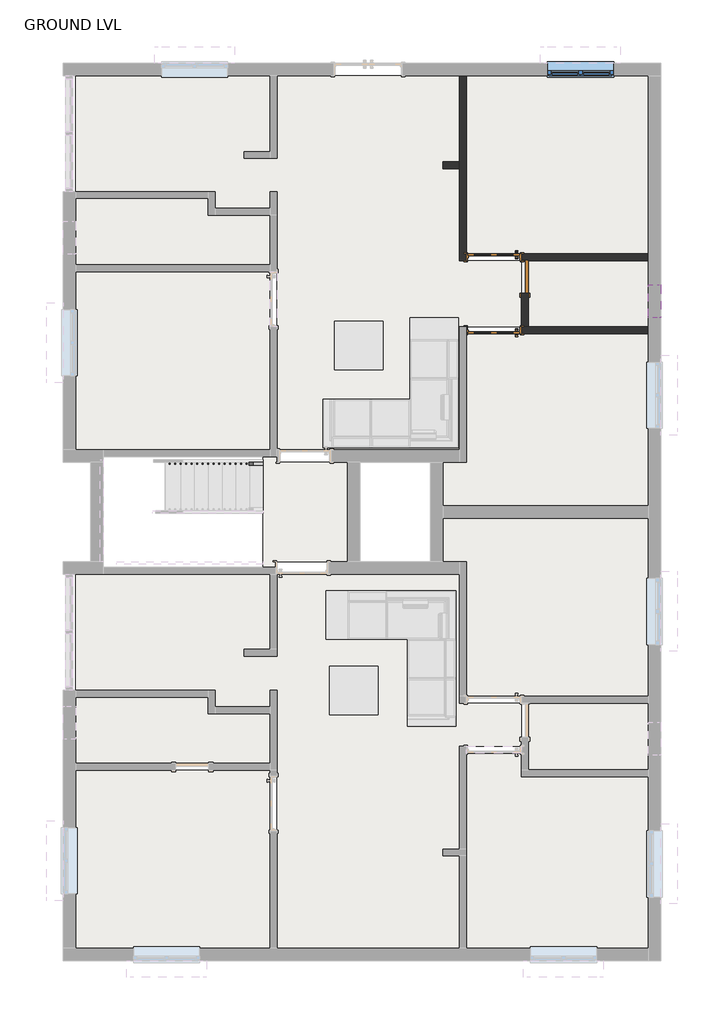
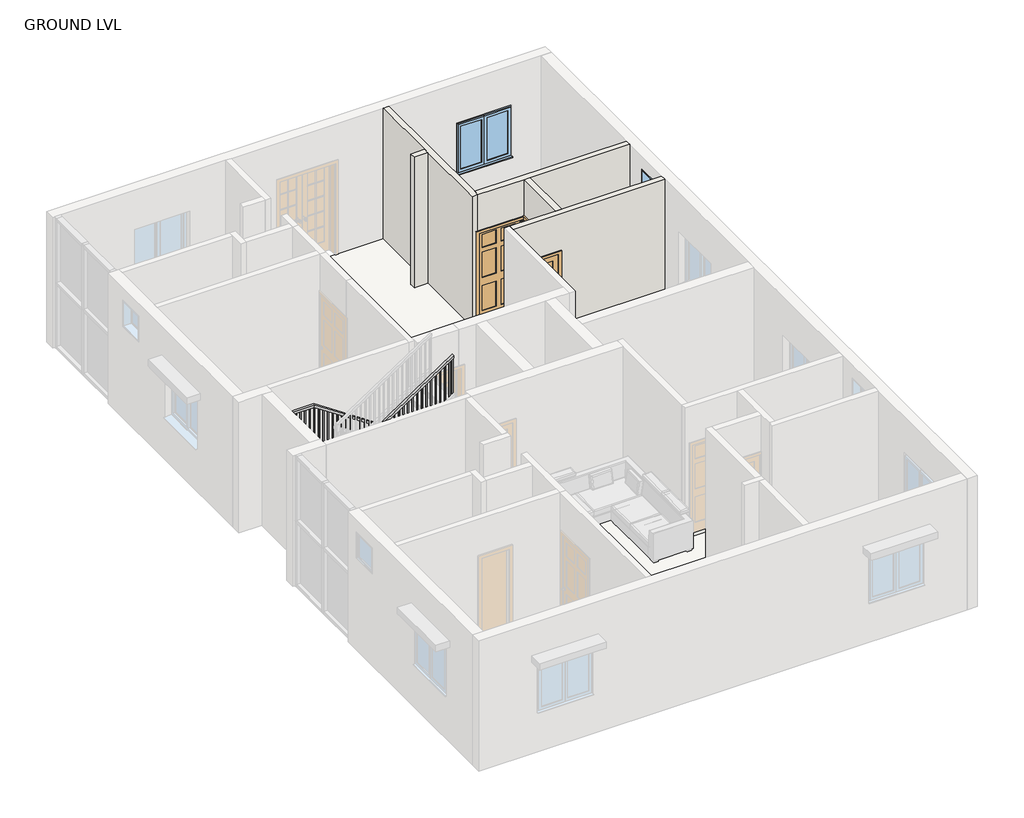
# One storey, part 3 of 4: 5 walls, 4 slabs, 3 doors, 2 windows, 1 railing.
"""IFC4 building model written with IfcOpenShell, lengths in millimetres."""

from ifc_helpers import new_model, si_unit, frame, origin, place, context, project, spatial, polyline, outline, extrude, faceted_brep, transform, mapped, element, save
from components import door_6a452240, door_3d68aebc, single_flush_flush_door_2_x_7_931cabab, window_80340324, w2_windows_4_x_4_9dec5fc7

model = new_model("IFC4")

# Units and contexts
model_context = context("Model", 3, world=origin())
ifc_project = project(units=[si_unit("LENGTHUNIT", "METRE", prefix="MILLI")], contexts=[model_context])

# Site, building, storey
site = spatial("IfcSite", under=ifc_project)
building = spatial("IfcBuilding", under=site)
storey = spatial("IfcBuildingStorey", under=building, Name="GROUND LVL", Elevation=3048.0)

# Doors
placement = place(None, origin())
door_shape = door_6a452240(model_context)
element("IfcDoor", 1, ObjectType="Door-Interior-Single-6_Panel-Wood : interior door 3' 4\" x 7'", at=placement, inside=storey, context=model_context, shape_type="MappedRepresentation", body=[
    mapped(door_shape, transform((1493.7987798, 9705.7059003, 3048.0), x_axis=(-1.0, 0.0, 0.0), y_axis=(0.0, -1.0, 0.0), z_axis=(0.0, 0.0, 1.0))),
])
door_2_shape = door_3d68aebc(model_context)
element("IfcDoor", 2, ObjectType="Door-Interior-Single-6_Panel-Wood : interior door 3' 4\" x 7'", at=placement, inside=storey, context=model_context, shape_type="MappedRepresentation", body=[
    mapped(door_2_shape, transform((1493.7987798, 8353.1559003, 3048.0), x_axis=(-1.0, 0.0, 0.0), y_axis=(0.0, -1.0, 0.0), z_axis=(0.0, 0.0, 1.0))),
])
single_flush_flush_door_2_x_7_shape = single_flush_flush_door_2_x_7_931cabab(model_context)
element("IfcDoor", 3, ObjectType="Single-Flush : flush door 2' x 7'", at=placement, inside=storey, context=model_context, shape_type="MappedRepresentation", body=[
    mapped(single_flush_flush_door_2_x_7_shape, transform((2065.2987798, 9346.9309003, 3048.0), x_axis=(0.0, 1.0, 0.0), y_axis=(-1.0, 0.0, 0.0), z_axis=(0.0, 0.0, 1.0))),
])

# Railing
element("IfcRailing", 4, ObjectType="Handrail - Rectangular", at=placement, inside=storey, context=model_context, shape_type="SolidModel", body=[
    faceted_brep([(-2748.0012202, 5879.8309003, 4131.7333333), (-2748.0012202, 5879.8309003, 4070.6793317), (-2748.0012202, 5930.6309003, 4070.6793317), (-2748.0012202, 5930.6309003, 4131.7333333), (-4780.0012202, 5879.8309003, 5486.4), (-4795.3822226, 5879.8309003, 5435.6), (-4795.3822226, 5930.6309003, 5435.6), (-4780.0012202, 5930.6309003, 5486.4), (-5643.6012202, 5879.8309003, 5486.4), (-5643.6012202, 5879.8309003, 5435.6), (-5694.4012202, 5930.6309003, 5435.6), (-5694.4012202, 5930.6309003, 5486.4), (-5643.6012202, 4152.6309003, 5486.4), (-5643.6012202, 4152.6309003, 5435.6), (-5694.4012202, 4101.8309003, 5435.6), (-5694.4012202, 4101.8309003, 5486.4), (-5034.0012202, 4152.6309003, 5486.4), (-5018.6202178, 4152.6309003, 5435.6), (-5018.6202178, 4101.8309003, 5435.6), (-5034.0012202, 4101.8309003, 5486.4), (-2748.0012202, 4152.6309003, 7010.4), (-2748.0012202, 4101.8309003, 7010.4), (-2748.0012202, 4101.8309003, 6949.3459984), (-2748.0012202, 4152.6309003, 6949.3459984)], [[[0, 1, 2, 3]], [[1, 0, 4, 5]], [[2, 1, 5, 6]], [[3, 2, 6, 7]], [[0, 3, 7, 4]], [[5, 4, 8, 9]], [[6, 5, 9, 10]], [[7, 6, 10, 11]], [[4, 7, 11, 8]], [[9, 8, 12, 13]], [[10, 9, 13, 14]], [[11, 10, 14, 15]], [[8, 11, 15, 12]], [[13, 12, 16, 17]], [[14, 13, 17, 18]], [[15, 14, 18, 19]], [[12, 15, 19, 16]], [[20, 21, 22, 23]], [[17, 16, 20, 23]], [[18, 17, 23, 22]], [[19, 18, 22, 21]], [[16, 19, 21, 20]]]),
    extrude(outline(polyline([(6904.8959984, -2814.6762202), (6892.1959984, -2833.7262202), (5926.6666667, -2833.7262202), (5926.6666667, -2814.6762202), (6904.8959984, -2814.6762202)])), frame((0.0, 4117.7059003, 0.0), z_axis=(0.0, 1.0, 0.0), x_axis=(0.0, 0.0, 1.0)), (0.0, 0.0, 1.0), 19.05),
    extrude(outline(polyline([(6837.1626651, -2916.2762202), (6824.4626651, -2935.3262202), (5926.6666667, -2935.3262202), (5926.6666667, -2916.2762202), (6837.1626651, -2916.2762202)])), frame((0.0, 4117.7059003, 0.0), z_axis=(0.0, 1.0, 0.0), x_axis=(0.0, 0.0, 1.0)), (0.0, 0.0, 1.0), 19.05),
    extrude(outline(polyline([(6769.4293317, -3017.8762202), (6756.7293317, -3036.9262202), (5757.3333333, -3036.9262202), (5757.3333333, -3017.8762202), (6769.4293317, -3017.8762202)])), frame((0.0, 4117.7059003, 0.0), z_axis=(0.0, 1.0, 0.0), x_axis=(0.0, 0.0, 1.0)), (0.0, 0.0, 1.0), 19.05),
    extrude(outline(polyline([(6701.6959984, -3119.4762202), (6688.9959984, -3138.5262202), (5757.3333333, -3138.5262202), (5757.3333333, -3119.4762202), (6701.6959984, -3119.4762202)])), frame((0.0, 4117.7059003, 0.0), z_axis=(0.0, 1.0, 0.0), x_axis=(0.0, 0.0, 1.0)), (0.0, 0.0, 1.0), 19.05),
    extrude(outline(polyline([(6633.9626651, -3221.0762202), (6621.2626651, -3240.1262202), (5757.3333333, -3240.1262202), (5757.3333333, -3221.0762202), (6633.9626651, -3221.0762202)])), frame((0.0, 4117.7059003, 0.0), z_axis=(0.0, 1.0, 0.0), x_axis=(0.0, 0.0, 1.0)), (0.0, 0.0, 1.0), 19.05),
    extrude(outline(polyline([(6566.2293317, -3322.6762202), (6553.5293317, -3341.7262202), (5588.0, -3341.7262202), (5588.0, -3322.6762202), (6566.2293317, -3322.6762202)])), frame((0.0, 4117.7059003, 0.0), z_axis=(0.0, 1.0, 0.0), x_axis=(0.0, 0.0, 1.0)), (0.0, 0.0, 1.0), 19.05),
    extrude(outline(polyline([(6498.4959984, -3424.2762202), (6485.7959984, -3443.3262202), (5588.0, -3443.3262202), (5588.0, -3424.2762202), (6498.4959984, -3424.2762202)])), frame((0.0, 4117.7059003, 0.0), z_axis=(0.0, 1.0, 0.0), x_axis=(0.0, 0.0, 1.0)), (0.0, 0.0, 1.0), 19.05),
    extrude(outline(polyline([(6430.7626651, -3525.8762202), (6418.0626651, -3544.9262202), (5418.6666667, -3544.9262202), (5418.6666667, -3525.8762202), (6430.7626651, -3525.8762202)])), frame((0.0, 4117.7059003, 0.0), z_axis=(0.0, 1.0, 0.0), x_axis=(0.0, 0.0, 1.0)), (0.0, 0.0, 1.0), 19.05),
    extrude(outline(polyline([(6363.0293317, -3627.4762202), (6350.3293317, -3646.5262202), (5418.6666667, -3646.5262202), (5418.6666667, -3627.4762202), (6363.0293317, -3627.4762202)])), frame((0.0, 4117.7059003, 0.0), z_axis=(0.0, 1.0, 0.0), x_axis=(0.0, 0.0, 1.0)), (0.0, 0.0, 1.0), 19.05),
    extrude(outline(polyline([(6295.2959984, -3729.0762202), (6282.5959984, -3748.1262202), (5418.6666667, -3748.1262202), (5418.6666667, -3729.0762202), (6295.2959984, -3729.0762202)])), frame((0.0, 4117.7059003, 0.0), z_axis=(0.0, 1.0, 0.0), x_axis=(0.0, 0.0, 1.0)), (0.0, 0.0, 1.0), 19.05),
    extrude(outline(polyline([(6227.5626651, -3830.6762202), (6214.8626651, -3849.7262202), (5249.3333333, -3849.7262202), (5249.3333333, -3830.6762202), (6227.5626651, -3830.6762202)])), frame((0.0, 4117.7059003, 0.0), z_axis=(0.0, 1.0, 0.0), x_axis=(0.0, 0.0, 1.0)), (0.0, 0.0, 1.0), 19.05),
    extrude(outline(polyline([(6159.8293317, -3932.2762202), (6147.1293317, -3951.3262202), (5249.3333333, -3951.3262202), (5249.3333333, -3932.2762202), (6159.8293317, -3932.2762202)])), frame((0.0, 4117.7059003, 0.0), z_axis=(0.0, 1.0, 0.0), x_axis=(0.0, 0.0, 1.0)), (0.0, 0.0, 1.0), 19.05),
    extrude(outline(polyline([(6092.0959984, -4033.8762202), (6079.3959984, -4052.9262202), (5080.0, -4052.9262202), (5080.0, -4033.8762202), (6092.0959984, -4033.8762202)])), frame((0.0, 4117.7059003, 0.0), z_axis=(0.0, 1.0, 0.0), x_axis=(0.0, 0.0, 1.0)), (0.0, 0.0, 1.0), 19.05),
    extrude(outline(polyline([(6024.3626651, -4135.4762202), (6011.6626651, -4154.5262202), (5080.0, -4154.5262202), (5080.0, -4135.4762202), (6024.3626651, -4135.4762202)])), frame((0.0, 4117.7059003, 0.0), z_axis=(0.0, 1.0, 0.0), x_axis=(0.0, 0.0, 1.0)), (0.0, 0.0, 1.0), 19.05),
    extrude(outline(polyline([(5956.6293317, -4237.0762202), (5943.9293317, -4256.1262202), (5080.0, -4256.1262202), (5080.0, -4237.0762202), (5956.6293317, -4237.0762202)])), frame((0.0, 4117.7059003, 0.0), z_axis=(0.0, 1.0, 0.0), x_axis=(0.0, 0.0, 1.0)), (0.0, 0.0, 1.0), 19.05),
    extrude(outline(polyline([(5888.8959984, -4338.6762202), (5876.1959984, -4357.7262202), (4910.6666667, -4357.7262202), (4910.6666667, -4338.6762202), (5888.8959984, -4338.6762202)])), frame((0.0, 4117.7059003, 0.0), z_axis=(0.0, 1.0, 0.0), x_axis=(0.0, 0.0, 1.0)), (0.0, 0.0, 1.0), 19.05),
    extrude(outline(polyline([(5821.1626651, -4440.2762202), (5808.4626651, -4459.3262202), (4910.6666667, -4459.3262202), (4910.6666667, -4440.2762202), (5821.1626651, -4440.2762202)])), frame((0.0, 4117.7059003, 0.0), z_axis=(0.0, 1.0, 0.0), x_axis=(0.0, 0.0, 1.0)), (0.0, 0.0, 1.0), 19.05),
    extrude(outline(polyline([(5753.4293317, -4541.8762202), (5740.7293317, -4560.9262202), (4741.3333333, -4560.9262202), (4741.3333333, -4541.8762202), (5753.4293317, -4541.8762202)])), frame((0.0, 4117.7059003, 0.0), z_axis=(0.0, 1.0, 0.0), x_axis=(0.0, 0.0, 1.0)), (0.0, 0.0, 1.0), 19.05),
    extrude(outline(polyline([(5685.6959984, -4643.4762202), (5672.9959984, -4662.5262202), (4741.3333333, -4662.5262202), (4741.3333333, -4643.4762202), (5685.6959984, -4643.4762202)])), frame((0.0, 4117.7059003, 0.0), z_axis=(0.0, 1.0, 0.0), x_axis=(0.0, 0.0, 1.0)), (0.0, 0.0, 1.0), 19.05),
    extrude(outline(polyline([(5617.9626651, -4745.0762202), (5605.2626651, -4764.1262202), (4741.3333333, -4764.1262202), (4741.3333333, -4745.0762202), (5617.9626651, -4745.0762202)])), frame((0.0, 4117.7059003, 0.0), z_axis=(0.0, 1.0, 0.0), x_axis=(0.0, 0.0, 1.0)), (0.0, 0.0, 1.0), 19.05),
    extrude(outline(polyline([(5550.2293317, -4846.6762202), (5537.5293317, -4865.7262202), (4572.0, -4865.7262202), (4572.0, -4846.6762202), (5550.2293317, -4846.6762202)])), frame((0.0, 4117.7059003, 0.0), z_axis=(0.0, 1.0, 0.0), x_axis=(0.0, 0.0, 1.0)), (0.0, 0.0, 1.0), 19.05),
    extrude(outline(polyline([(5482.4959984, -4948.2762202), (5469.7959984, -4967.3262202), (4572.0, -4967.3262202), (4572.0, -4948.2762202), (5482.4959984, -4948.2762202)])), frame((0.0, 4117.7059003, 0.0), z_axis=(0.0, 1.0, 0.0), x_axis=(0.0, 0.0, 1.0)), (0.0, 0.0, 1.0), 19.05),
    extrude(outline(polyline([(-5068.9262202, 4117.7059003), (-5068.9262202, 4136.7559003), (-5049.8762202, 4136.7559003), (-5049.8762202, 4117.7059003), (-5068.9262202, 4117.7059003)])), frame((0.0, 0.0, 4572.0), z_axis=(0.0, 0.0, 1.0), x_axis=(1.0, 0.0, 0.0)), (0.0, 0.0, 1.0), 863.6),
    extrude(outline(polyline([(-5170.5262202, 4117.7059003), (-5170.5262202, 4136.7559003), (-5151.4762202, 4136.7559003), (-5151.4762202, 4117.7059003), (-5170.5262202, 4117.7059003)])), frame((0.0, 0.0, 4572.0), z_axis=(0.0, 0.0, 1.0), x_axis=(1.0, 0.0, 0.0)), (0.0, 0.0, 1.0), 863.6),
    extrude(outline(polyline([(-5272.1262202, 4117.7059003), (-5272.1262202, 4136.7559003), (-5253.0762202, 4136.7559003), (-5253.0762202, 4117.7059003), (-5272.1262202, 4117.7059003)])), frame((0.0, 0.0, 4572.0), z_axis=(0.0, 0.0, 1.0), x_axis=(1.0, 0.0, 0.0)), (0.0, 0.0, 1.0), 863.6),
    extrude(outline(polyline([(-5373.7262202, 4117.7059003), (-5373.7262202, 4136.7559003), (-5354.6762202, 4136.7559003), (-5354.6762202, 4117.7059003), (-5373.7262202, 4117.7059003)])), frame((0.0, 0.0, 4572.0), z_axis=(0.0, 0.0, 1.0), x_axis=(1.0, 0.0, 0.0)), (0.0, 0.0, 1.0), 863.6),
    extrude(outline(polyline([(-5475.3262202, 4117.7059003), (-5475.3262202, 4136.7559003), (-5456.2762202, 4136.7559003), (-5456.2762202, 4117.7059003), (-5475.3262202, 4117.7059003)])), frame((0.0, 0.0, 4572.0), z_axis=(0.0, 0.0, 1.0), x_axis=(1.0, 0.0, 0.0)), (0.0, 0.0, 1.0), 863.6),
    extrude(outline(polyline([(-5576.9262202, 4117.7059003), (-5576.9262202, 4136.7559003), (-5557.8762202, 4136.7559003), (-5557.8762202, 4117.7059003), (-5576.9262202, 4117.7059003)])), frame((0.0, 0.0, 4572.0), z_axis=(0.0, 0.0, 1.0), x_axis=(1.0, 0.0, 0.0)), (0.0, 0.0, 1.0), 863.6),
    extrude(outline(polyline([(-5678.5262202, 4187.5559003), (-5659.4762202, 4187.5559003), (-5659.4762202, 4168.5059003), (-5678.5262202, 4168.5059003), (-5678.5262202, 4187.5559003)])), frame((0.0, 0.0, 4572.0), z_axis=(0.0, 0.0, 1.0), x_axis=(1.0, 0.0, 0.0)), (0.0, 0.0, 1.0), 863.6),
    extrude(outline(polyline([(-5678.5262202, 4289.1559003), (-5659.4762202, 4289.1559003), (-5659.4762202, 4270.1059003), (-5678.5262202, 4270.1059003), (-5678.5262202, 4289.1559003)])), frame((0.0, 0.0, 4572.0), z_axis=(0.0, 0.0, 1.0), x_axis=(1.0, 0.0, 0.0)), (0.0, 0.0, 1.0), 863.6),
    extrude(outline(polyline([(-5678.5262202, 4390.7559003), (-5659.4762202, 4390.7559003), (-5659.4762202, 4371.7059003), (-5678.5262202, 4371.7059003), (-5678.5262202, 4390.7559003)])), frame((0.0, 0.0, 4572.0), z_axis=(0.0, 0.0, 1.0), x_axis=(1.0, 0.0, 0.0)), (0.0, 0.0, 1.0), 863.6),
    extrude(outline(polyline([(-5678.5262202, 4492.3559003), (-5659.4762202, 4492.3559003), (-5659.4762202, 4473.3059003), (-5678.5262202, 4473.3059003), (-5678.5262202, 4492.3559003)])), frame((0.0, 0.0, 4572.0), z_axis=(0.0, 0.0, 1.0), x_axis=(1.0, 0.0, 0.0)), (0.0, 0.0, 1.0), 863.6),
    extrude(outline(polyline([(-5678.5262202, 4593.9559003), (-5659.4762202, 4593.9559003), (-5659.4762202, 4574.9059003), (-5678.5262202, 4574.9059003), (-5678.5262202, 4593.9559003)])), frame((0.0, 0.0, 4572.0), z_axis=(0.0, 0.0, 1.0), x_axis=(1.0, 0.0, 0.0)), (0.0, 0.0, 1.0), 863.6),
    extrude(outline(polyline([(-5678.5262202, 4695.5559003), (-5659.4762202, 4695.5559003), (-5659.4762202, 4676.5059003), (-5678.5262202, 4676.5059003), (-5678.5262202, 4695.5559003)])), frame((0.0, 0.0, 4572.0), z_axis=(0.0, 0.0, 1.0), x_axis=(1.0, 0.0, 0.0)), (0.0, 0.0, 1.0), 863.6),
    extrude(outline(polyline([(-5678.5262202, 4797.1559003), (-5659.4762202, 4797.1559003), (-5659.4762202, 4778.1059003), (-5678.5262202, 4778.1059003), (-5678.5262202, 4797.1559003)])), frame((0.0, 0.0, 4572.0), z_axis=(0.0, 0.0, 1.0), x_axis=(1.0, 0.0, 0.0)), (0.0, 0.0, 1.0), 863.6),
    extrude(outline(polyline([(-5678.5262202, 4898.7559003), (-5659.4762202, 4898.7559003), (-5659.4762202, 4879.7059003), (-5678.5262202, 4879.7059003), (-5678.5262202, 4898.7559003)])), frame((0.0, 0.0, 4572.0), z_axis=(0.0, 0.0, 1.0), x_axis=(1.0, 0.0, 0.0)), (0.0, 0.0, 1.0), 863.6),
    extrude(outline(polyline([(-5678.5262202, 5000.3559003), (-5659.4762202, 5000.3559003), (-5659.4762202, 4981.3059003), (-5678.5262202, 4981.3059003), (-5678.5262202, 5000.3559003)])), frame((0.0, 0.0, 4572.0), z_axis=(0.0, 0.0, 1.0), x_axis=(1.0, 0.0, 0.0)), (0.0, 0.0, 1.0), 863.6),
    extrude(outline(polyline([(-5678.5262202, 5101.9559003), (-5659.4762202, 5101.9559003), (-5659.4762202, 5082.9059003), (-5678.5262202, 5082.9059003), (-5678.5262202, 5101.9559003)])), frame((0.0, 0.0, 4572.0), z_axis=(0.0, 0.0, 1.0), x_axis=(1.0, 0.0, 0.0)), (0.0, 0.0, 1.0), 863.6),
    extrude(outline(polyline([(-5678.5262202, 5203.5559003), (-5659.4762202, 5203.5559003), (-5659.4762202, 5184.5059003), (-5678.5262202, 5184.5059003), (-5678.5262202, 5203.5559003)])), frame((0.0, 0.0, 4572.0), z_axis=(0.0, 0.0, 1.0), x_axis=(1.0, 0.0, 0.0)), (0.0, 0.0, 1.0), 863.6),
    extrude(outline(polyline([(-5678.5262202, 5305.1559003), (-5659.4762202, 5305.1559003), (-5659.4762202, 5286.1059003), (-5678.5262202, 5286.1059003), (-5678.5262202, 5305.1559003)])), frame((0.0, 0.0, 4572.0), z_axis=(0.0, 0.0, 1.0), x_axis=(1.0, 0.0, 0.0)), (0.0, 0.0, 1.0), 863.6),
    extrude(outline(polyline([(-5678.5262202, 5406.7559003), (-5659.4762202, 5406.7559003), (-5659.4762202, 5387.7059003), (-5678.5262202, 5387.7059003), (-5678.5262202, 5406.7559003)])), frame((0.0, 0.0, 4572.0), z_axis=(0.0, 0.0, 1.0), x_axis=(1.0, 0.0, 0.0)), (0.0, 0.0, 1.0), 863.6),
    extrude(outline(polyline([(-5678.5262202, 5508.3559003), (-5659.4762202, 5508.3559003), (-5659.4762202, 5489.3059003), (-5678.5262202, 5489.3059003), (-5678.5262202, 5508.3559003)])), frame((0.0, 0.0, 4572.0), z_axis=(0.0, 0.0, 1.0), x_axis=(1.0, 0.0, 0.0)), (0.0, 0.0, 1.0), 863.6),
    extrude(outline(polyline([(-5678.5262202, 5609.9559003), (-5659.4762202, 5609.9559003), (-5659.4762202, 5590.9059003), (-5678.5262202, 5590.9059003), (-5678.5262202, 5609.9559003)])), frame((0.0, 0.0, 4572.0), z_axis=(0.0, 0.0, 1.0), x_axis=(1.0, 0.0, 0.0)), (0.0, 0.0, 1.0), 863.6),
    extrude(outline(polyline([(-5678.5262202, 5711.5559003), (-5659.4762202, 5711.5559003), (-5659.4762202, 5692.5059003), (-5678.5262202, 5692.5059003), (-5678.5262202, 5711.5559003)])), frame((0.0, 0.0, 4572.0), z_axis=(0.0, 0.0, 1.0), x_axis=(1.0, 0.0, 0.0)), (0.0, 0.0, 1.0), 863.6),
    extrude(outline(polyline([(-5678.5262202, 5813.1559003), (-5659.4762202, 5813.1559003), (-5659.4762202, 5794.1059003), (-5678.5262202, 5794.1059003), (-5678.5262202, 5813.1559003)])), frame((0.0, 0.0, 4572.0), z_axis=(0.0, 0.0, 1.0), x_axis=(1.0, 0.0, 0.0)), (0.0, 0.0, 1.0), 863.6),
    extrude(outline(polyline([(-5583.2762202, 5914.7559003), (-5583.2762202, 5895.7059003), (-5602.3262202, 5895.7059003), (-5602.3262202, 5914.7559003), (-5583.2762202, 5914.7559003)])), frame((0.0, 0.0, 4572.0), z_axis=(0.0, 0.0, 1.0), x_axis=(1.0, 0.0, 0.0)), (0.0, 0.0, 1.0), 863.6),
    extrude(outline(polyline([(-5481.6762202, 5914.7559003), (-5481.6762202, 5895.7059003), (-5500.7262202, 5895.7059003), (-5500.7262202, 5914.7559003), (-5481.6762202, 5914.7559003)])), frame((0.0, 0.0, 4572.0), z_axis=(0.0, 0.0, 1.0), x_axis=(1.0, 0.0, 0.0)), (0.0, 0.0, 1.0), 863.6),
    extrude(outline(polyline([(-5380.0762202, 5914.7559003), (-5380.0762202, 5895.7059003), (-5399.1262202, 5895.7059003), (-5399.1262202, 5914.7559003), (-5380.0762202, 5914.7559003)])), frame((0.0, 0.0, 4572.0), z_axis=(0.0, 0.0, 1.0), x_axis=(1.0, 0.0, 0.0)), (0.0, 0.0, 1.0), 863.6),
    extrude(outline(polyline([(-5278.4762202, 5914.7559003), (-5278.4762202, 5895.7059003), (-5297.5262202, 5895.7059003), (-5297.5262202, 5914.7559003), (-5278.4762202, 5914.7559003)])), frame((0.0, 0.0, 4572.0), z_axis=(0.0, 0.0, 1.0), x_axis=(1.0, 0.0, 0.0)), (0.0, 0.0, 1.0), 863.6),
    extrude(outline(polyline([(-5176.8762202, 5914.7559003), (-5176.8762202, 5895.7059003), (-5195.9262202, 5895.7059003), (-5195.9262202, 5914.7559003), (-5176.8762202, 5914.7559003)])), frame((0.0, 0.0, 4572.0), z_axis=(0.0, 0.0, 1.0), x_axis=(1.0, 0.0, 0.0)), (0.0, 0.0, 1.0), 863.6),
    extrude(outline(polyline([(-5075.2762202, 5914.7559003), (-5075.2762202, 5895.7059003), (-5094.3262202, 5895.7059003), (-5094.3262202, 5914.7559003), (-5075.2762202, 5914.7559003)])), frame((0.0, 0.0, 4572.0), z_axis=(0.0, 0.0, 1.0), x_axis=(1.0, 0.0, 0.0)), (0.0, 0.0, 1.0), 863.6),
    extrude(outline(polyline([(-4973.6762202, 5914.7559003), (-4973.6762202, 5895.7059003), (-4992.7262202, 5895.7059003), (-4992.7262202, 5914.7559003), (-4973.6762202, 5914.7559003)])), frame((0.0, 0.0, 4572.0), z_axis=(0.0, 0.0, 1.0), x_axis=(1.0, 0.0, 0.0)), (0.0, 0.0, 1.0), 863.6),
    extrude(outline(polyline([(-4872.0762202, 5914.7559003), (-4872.0762202, 5895.7059003), (-4891.1262202, 5895.7059003), (-4891.1262202, 5914.7559003), (-4872.0762202, 5914.7559003)])), frame((0.0, 0.0, 4572.0), z_axis=(0.0, 0.0, 1.0), x_axis=(1.0, 0.0, 0.0)), (0.0, 0.0, 1.0), 863.6),
    extrude(outline(polyline([(5418.9959984, -4770.4762202), (5431.6959984, -4789.5262202), (4572.0, -4789.5262202), (4572.0, -4770.4762202), (5418.9959984, -4770.4762202)])), frame((0.0, 5895.7059003, 0.0), z_axis=(0.0, 1.0, 0.0), x_axis=(0.0, 0.0, 1.0)), (0.0, 0.0, 1.0), 19.05),
    extrude(outline(polyline([(5351.2626651, -4668.8762202), (5363.9626651, -4687.9262202), (4402.6666667, -4687.9262202), (4402.6666667, -4668.8762202), (5351.2626651, -4668.8762202)])), frame((0.0, 5895.7059003, 0.0), z_axis=(0.0, 1.0, 0.0), x_axis=(0.0, 0.0, 1.0)), (0.0, 0.0, 1.0), 19.05),
    extrude(outline(polyline([(5283.5293317, -4567.2762202), (5296.2293317, -4586.3262202), (4402.6666667, -4586.3262202), (4402.6666667, -4567.2762202), (5283.5293317, -4567.2762202)])), frame((0.0, 5895.7059003, 0.0), z_axis=(0.0, 1.0, 0.0), x_axis=(0.0, 0.0, 1.0)), (0.0, 0.0, 1.0), 19.05),
    extrude(outline(polyline([(5215.7959984, -4465.6762202), (5228.4959984, -4484.7262202), (4233.3333333, -4484.7262202), (4233.3333333, -4465.6762202), (5215.7959984, -4465.6762202)])), frame((0.0, 5895.7059003, 0.0), z_axis=(0.0, 1.0, 0.0), x_axis=(0.0, 0.0, 1.0)), (0.0, 0.0, 1.0), 19.05),
    extrude(outline(polyline([(5148.0626651, -4364.0762202), (5160.7626651, -4383.1262202), (4233.3333333, -4383.1262202), (4233.3333333, -4364.0762202), (5148.0626651, -4364.0762202)])), frame((0.0, 5895.7059003, 0.0), z_axis=(0.0, 1.0, 0.0), x_axis=(0.0, 0.0, 1.0)), (0.0, 0.0, 1.0), 19.05),
    extrude(outline(polyline([(5080.3293317, -4262.4762202), (5093.0293317, -4281.5262202), (4233.3333333, -4281.5262202), (4233.3333333, -4262.4762202), (5080.3293317, -4262.4762202)])), frame((0.0, 5895.7059003, 0.0), z_axis=(0.0, 1.0, 0.0), x_axis=(0.0, 0.0, 1.0)), (0.0, 0.0, 1.0), 19.05),
    extrude(outline(polyline([(5012.5959984, -4160.8762202), (5025.2959984, -4179.9262202), (4064.0, -4179.9262202), (4064.0, -4160.8762202), (5012.5959984, -4160.8762202)])), frame((0.0, 5895.7059003, 0.0), z_axis=(0.0, 1.0, 0.0), x_axis=(0.0, 0.0, 1.0)), (0.0, 0.0, 1.0), 19.05),
    extrude(outline(polyline([(4944.8626651, -4059.2762202), (4957.5626651, -4078.3262202), (4064.0, -4078.3262202), (4064.0, -4059.2762202), (4944.8626651, -4059.2762202)])), frame((0.0, 5895.7059003, 0.0), z_axis=(0.0, 1.0, 0.0), x_axis=(0.0, 0.0, 1.0)), (0.0, 0.0, 1.0), 19.05),
    extrude(outline(polyline([(4877.1293317, -3957.6762202), (4889.8293317, -3976.7262202), (3894.6666667, -3976.7262202), (3894.6666667, -3957.6762202), (4877.1293317, -3957.6762202)])), frame((0.0, 5895.7059003, 0.0), z_axis=(0.0, 1.0, 0.0), x_axis=(0.0, 0.0, 1.0)), (0.0, 0.0, 1.0), 19.05),
    extrude(outline(polyline([(4809.3959984, -3856.0762202), (4822.0959984, -3875.1262202), (3894.6666667, -3875.1262202), (3894.6666667, -3856.0762202), (4809.3959984, -3856.0762202)])), frame((0.0, 5895.7059003, 0.0), z_axis=(0.0, 1.0, 0.0), x_axis=(0.0, 0.0, 1.0)), (0.0, 0.0, 1.0), 19.05),
    extrude(outline(polyline([(4741.6626651, -3754.4762202), (4754.3626651, -3773.5262202), (3894.6666667, -3773.5262202), (3894.6666667, -3754.4762202), (4741.6626651, -3754.4762202)])), frame((0.0, 5895.7059003, 0.0), z_axis=(0.0, 1.0, 0.0), x_axis=(0.0, 0.0, 1.0)), (0.0, 0.0, 1.0), 19.05),
    extrude(outline(polyline([(4673.9293317, -3652.8762202), (4686.6293317, -3671.9262202), (3725.3333333, -3671.9262202), (3725.3333333, -3652.8762202), (4673.9293317, -3652.8762202)])), frame((0.0, 5895.7059003, 0.0), z_axis=(0.0, 1.0, 0.0), x_axis=(0.0, 0.0, 1.0)), (0.0, 0.0, 1.0), 19.05),
    extrude(outline(polyline([(4606.1959984, -3551.2762202), (4618.8959984, -3570.3262202), (3725.3333333, -3570.3262202), (3725.3333333, -3551.2762202), (4606.1959984, -3551.2762202)])), frame((0.0, 5895.7059003, 0.0), z_axis=(0.0, 1.0, 0.0), x_axis=(0.0, 0.0, 1.0)), (0.0, 0.0, 1.0), 19.05),
    extrude(outline(polyline([(4538.4626651, -3449.6762202), (4551.1626651, -3468.7262202), (3556.0, -3468.7262202), (3556.0, -3449.6762202), (4538.4626651, -3449.6762202)])), frame((0.0, 5895.7059003, 0.0), z_axis=(0.0, 1.0, 0.0), x_axis=(0.0, 0.0, 1.0)), (0.0, 0.0, 1.0), 19.05),
    extrude(outline(polyline([(4470.7293317, -3348.0762202), (4483.4293317, -3367.1262202), (3556.0, -3367.1262202), (3556.0, -3348.0762202), (4470.7293317, -3348.0762202)])), frame((0.0, 5895.7059003, 0.0), z_axis=(0.0, 1.0, 0.0), x_axis=(0.0, 0.0, 1.0)), (0.0, 0.0, 1.0), 19.05),
    extrude(outline(polyline([(4402.9959984, -3246.4762202), (4415.6959984, -3265.5262202), (3556.0, -3265.5262202), (3556.0, -3246.4762202), (4402.9959984, -3246.4762202)])), frame((0.0, 5895.7059003, 0.0), z_axis=(0.0, 1.0, 0.0), x_axis=(0.0, 0.0, 1.0)), (0.0, 0.0, 1.0), 19.05),
    extrude(outline(polyline([(4335.2626651, -3144.8762202), (4347.9626651, -3163.9262202), (3386.6666667, -3163.9262202), (3386.6666667, -3144.8762202), (4335.2626651, -3144.8762202)])), frame((0.0, 5895.7059003, 0.0), z_axis=(0.0, 1.0, 0.0), x_axis=(0.0, 0.0, 1.0)), (0.0, 0.0, 1.0), 19.05),
    extrude(outline(polyline([(4267.5293317, -3043.2762202), (4280.2293317, -3062.3262202), (3386.6666667, -3062.3262202), (3386.6666667, -3043.2762202), (4267.5293317, -3043.2762202)])), frame((0.0, 5895.7059003, 0.0), z_axis=(0.0, 1.0, 0.0), x_axis=(0.0, 0.0, 1.0)), (0.0, 0.0, 1.0), 19.05),
    extrude(outline(polyline([(4199.7959984, -2941.6762202), (4212.4959984, -2960.7262202), (3217.3333333, -2960.7262202), (3217.3333333, -2941.6762202), (4199.7959984, -2941.6762202)])), frame((0.0, 5895.7059003, 0.0), z_axis=(0.0, 1.0, 0.0), x_axis=(0.0, 0.0, 1.0)), (0.0, 0.0, 1.0), 19.05),
    extrude(outline(polyline([(4132.0626651, -2840.0762202), (4144.7626651, -2859.1262202), (3217.3333333, -2859.1262202), (3217.3333333, -2840.0762202), (4132.0626651, -2840.0762202)])), frame((0.0, 5895.7059003, 0.0), z_axis=(0.0, 1.0, 0.0), x_axis=(0.0, 0.0, 1.0)), (0.0, 0.0, 1.0), 19.05),
    extrude(outline(polyline([(-5678.5262202, 4136.7559003), (-5659.4762202, 4136.7559003), (-5659.4762202, 4117.7059003), (-5678.5262202, 4117.7059003), (-5678.5262202, 4136.7559003)])), frame((0.0, 0.0, 4572.0), z_axis=(0.0, 0.0, 1.0), x_axis=(1.0, 0.0, 0.0)), (0.0, 0.0, 1.0), 863.6),
    extrude(outline(polyline([(-5659.4762202, 5914.7559003), (-5659.4762202, 5895.7059003), (-5678.5262202, 5895.7059003), (-5678.5262202, 5914.7559003), (-5659.4762202, 5914.7559003)])), frame((0.0, 0.0, 4572.0), z_axis=(0.0, 0.0, 1.0), x_axis=(1.0, 0.0, 0.0)), (0.0, 0.0, 1.0), 863.6),
    extrude(outline(polyline([(6949.3459984, -2748.0012202), (6936.6459984, -2767.0512202), (5926.6666667, -2767.0512202), (5926.6666667, -2748.0012202), (6949.3459984, -2748.0012202)])), frame((0.0, 4117.7059003, 0.0), z_axis=(0.0, 1.0, 0.0), x_axis=(0.0, 0.0, 1.0)), (0.0, 0.0, 1.0), 19.05),
    extrude(outline(polyline([(4070.6793317, -2748.0012202), (4083.3793317, -2767.0512202), (3217.3333333, -2767.0512202), (3217.3333333, -2748.0012202), (4070.6793317, -2748.0012202)])), frame((0.0, 5895.7059003, 0.0), z_axis=(0.0, 1.0, 0.0), x_axis=(0.0, 0.0, 1.0)), (0.0, 0.0, 1.0), 19.05),
])

# Slabs
element("IfcSlab", 5, ObjectType="FLOORING 6\"", at=placement, inside=storey, context=model_context, shape_type="SweptSolid", body=[
    extrude(outline(polyline([(-2621.0012202, 11645.6309003), (-3103.6012202, 11645.6309003), (-3103.6012202, 11518.6309003), (-2557.5012202, 11518.6309003), (-2494.0012202, 11518.6309003), (-2494.0012202, 13042.6309003), (858.7987798, 13042.6309003), (858.7987798, 11455.1309003), (553.9987798, 11455.1309003), (553.9987798, 11328.1309003), (858.7987798, 11328.1309003), (858.7987798, 9639.0309003), (2001.7987798, 9639.0309003), (2001.7987798, 8419.8309003), (858.7987798, 8419.8309003), (858.7987798, 6159.2309003), (-2494.0012202, 6159.2309003), (-2494.0012202, 9435.8309003), (-2494.0012202, 10909.0309003), (-2621.0012202, 10909.0309003), (-2621.0012202, 10604.2309003), (-3637.0012202, 10604.2309003), (-3637.0012202, 10909.0309003), (-6202.4012202, 10909.0309003), (-6202.4012202, 13042.6309003), (-2621.0012202, 13042.6309003), (-2621.0012202, 11645.6309003)])), frame((0.0, 0.0, 2895.6), z_axis=(0.0, 0.0, 1.0), x_axis=(1.0, 0.0, 0.0)), (0.0, 0.0, 1.0), 152.4),
])
element("IfcSlab", 6, ObjectType="FLOORING 6\"", at=placement, inside=storey, context=model_context, shape_type="SweptSolid", body=[
    extrude(outline(polyline([(4338.5987798, 13042.6309003), (4338.5987798, 9766.0309003), (985.7987798, 9766.0309003), (985.7987798, 13042.6309003), (4338.5987798, 13042.6309003)])), frame((0.0, 0.0, 2895.6), z_axis=(0.0, 0.0, 1.0), x_axis=(1.0, 0.0, 0.0)), (0.0, 0.0, 1.0), 152.4),
    extrude(outline(polyline([(4338.5987798, 9639.0309003), (4338.5987798, 8419.8309003), (2128.7987798, 8419.8309003), (2128.7987798, 9639.0309003), (4338.5987798, 9639.0309003)])), frame((0.0, 0.0, 2895.6), z_axis=(0.0, 0.0, 1.0), x_axis=(1.0, 0.0, 0.0)), (0.0, 0.0, 1.0), 152.4),
    extrude(outline(polyline([(-2621.0012202, 9435.8309003), (-2621.0012202, 6159.2309003), (-6202.4012202, 6159.2309003), (-6202.4012202, 9435.8309003), (-2621.0012202, 9435.8309003)])), frame((0.0, 0.0, 2895.6), z_axis=(0.0, 0.0, 1.0), x_axis=(1.0, 0.0, 0.0)), (0.0, 0.0, 1.0), 152.4),
    extrude(outline(polyline([(-2621.0012202, 9562.8309003), (-6202.4012202, 9562.8309003), (-6202.4012202, 10782.0309003), (-3764.0012202, 10782.0309003), (-3764.0012202, 10477.2309003), (-2621.0012202, 10477.2309003), (-2621.0012202, 9562.8309003)])), frame((0.0, 0.0, 2895.6), z_axis=(0.0, 0.0, 1.0), x_axis=(1.0, 0.0, 0.0)), (0.0, 0.0, 1.0), 152.4),
    extrude(outline(polyline([(553.9987798, 5930.6309003), (985.7987798, 5930.6309003), (985.7987798, 8292.8309003), (4338.5987798, 8292.8309003), (4338.5987798, 5130.5309003), (553.9987798, 5130.5309003), (553.9987798, 5930.6309003)])), frame((0.0, 0.0, 2895.6), z_axis=(0.0, 0.0, 1.0), x_axis=(1.0, 0.0, 0.0)), (0.0, 0.0, 1.0), 152.4),
])
element("IfcSlab", 7, ObjectType="FLOORING 6\"", at=placement, inside=storey, context=model_context, shape_type="SweptSolid", body=[
    extrude(outline(polyline([(985.7987798, 583.9309003), (2001.7987798, 583.9309003), (2001.7987798, 152.1309003), (4338.5987798, 152.1309003), (4338.5987798, -3010.1690997), (985.7987798, -3010.1690997), (985.7987798, 583.9309003)])), frame((0.0, 0.0, 2895.6), z_axis=(0.0, 0.0, 1.0), x_axis=(1.0, 0.0, 0.0)), (0.0, 0.0, 1.0), 152.4),
    extrude(outline(polyline([(-6203.9887202, -3010.1690997), (-6203.9887202, 266.4309003), (-2621.0012202, 266.4309003), (-2621.0012202, -3010.1690997), (-6203.9887202, -3010.1690997)])), frame((0.0, 0.0, 2895.6), z_axis=(0.0, 0.0, 1.0), x_axis=(1.0, 0.0, 0.0)), (0.0, 0.0, 1.0), 152.4),
    extrude(outline(polyline([(-2621.0012202, 393.4309003), (-6203.9887202, 393.4309003), (-6203.9887202, 1612.6309003), (-3764.0012202, 1612.6309003), (-3764.0012202, 1307.8309003), (-2621.0012202, 1307.8309003), (-2621.0012202, 393.4309003)])), frame((0.0, 0.0, 2895.6), z_axis=(0.0, 0.0, 1.0), x_axis=(1.0, 0.0, 0.0)), (0.0, 0.0, 1.0), 152.4),
    extrude(outline(polyline([(858.7987798, -3010.1690997), (-2494.0012202, -3010.1690997), (-2494.0012202, 1739.6309003), (-2621.0012202, 1739.6309003), (-2621.0012202, 1434.8309003), (-3637.0012202, 1434.8309003), (-3637.0012202, 1739.6309003), (-6203.9887202, 1739.6309003), (-6203.9887202, 3873.2309003), (-2621.0012202, 3873.2309003), (-2621.0012202, 2488.9309003), (-3103.6012202, 2488.9309003), (-3103.6012202, 2361.9309003), (-2494.0012202, 2361.9309003), (-2494.0012202, 3873.2309003), (858.7987798, 3873.2309003), (858.7987798, 1498.3309003), (2001.7987798, 1498.3309003), (2001.7987798, 710.9309003), (858.7987798, 710.9309003), (858.7987798, -3010.1690997)])), frame((0.0, 0.0, 2895.6), z_axis=(0.0, 0.0, 1.0), x_axis=(1.0, 0.0, 0.0)), (0.0, 0.0, 1.0), 152.4),
    extrude(outline(polyline([(985.7987798, 1625.3309003), (985.7987798, 4101.8309003), (553.9987798, 4101.8309003), (553.9987798, 4901.9309003), (4338.5987798, 4901.9309003), (4338.5987798, 1625.3309003), (985.7987798, 1625.3309003)])), frame((0.0, 0.0, 2895.6), z_axis=(0.0, 0.0, 1.0), x_axis=(1.0, 0.0, 0.0)), (0.0, 0.0, 1.0), 152.4),
    extrude(outline(polyline([(-2748.0012202, 4000.2309003), (-2748.0012202, 5981.4309003), (-2748.0012202, 6032.2309003), (-2494.0012202, 6032.2309003), (-2494.0012202, 5930.6309003), (-1198.6012202, 5930.6309003), (-1198.6012202, 4101.8309003), (-2494.0012202, 4101.8309003), (-2494.0012202, 4000.2309003), (-2748.0012202, 4000.2309003)])), frame((0.0, 0.0, 2895.6), z_axis=(0.0, 0.0, 1.0), x_axis=(1.0, 0.0, 0.0)), (0.0, 0.0, 1.0), 152.4),
])
element("IfcSlab", 8, ObjectType="bathroom tiles", at=placement, inside=storey, context=model_context, shape_type="SweptSolid", body=[
    extrude(outline(polyline([(4338.5987798, 1498.3309003), (4338.5987798, 279.1309003), (2128.7987798, 279.1309003), (2128.7987798, 1498.3309003), (4338.5987798, 1498.3309003)])), frame((0.0, 0.0, 2895.6), z_axis=(0.0, 0.0, 1.0), x_axis=(1.0, 0.0, 0.0)), (0.0, 0.0, 1.0), 152.4),
])

# Walls
element("IfcWall", 9, ObjectType="inner wall 5\"", at=placement, inside=storey, context=model_context, shape_type="Brep", body=[
    faceted_brep([(985.7987798, 9639.0309003, 3048.0), (985.7987798, 13042.6309003, 3048.0), (985.7987798, 13042.6309003, 6096.0), (985.7987798, 9766.0309003, 6096.0), (985.7987798, 9639.0309003, 6096.0), (985.7987798, 9639.0309003, 5207.0), (858.7987798, 9639.0309003, 3048.0), (858.7987798, 9639.0309003, 6096.0), (858.7987798, 11328.1309003, 6096.0), (858.7987798, 11455.1309003, 6096.0), (858.7987798, 13042.6309003, 6096.0), (858.7987798, 13042.6309003, 3048.0), (858.7987798, 11455.1309003, 3048.0), (858.7987798, 11328.1309003, 3048.0)], [[[0, 1, 2, 3, 4, 5]], [[6, 7, 8, 9, 10, 11, 12, 13]], [[1, 0, 6, 13, 12, 11]], [[4, 3, 2, 10, 9, 8, 7]], [[2, 1, 11, 10]], [[0, 5, 4, 7, 6]]]),
])
element("IfcWall", 10, ObjectType="inner wall 5\"", at=placement, inside=storey, context=model_context, shape_type="SweptSolid", body=[
    extrude(outline(polyline([(858.7987798, 11328.1309003), (553.9987798, 11328.1309003), (553.9987798, 11455.1309003), (858.7987798, 11455.1309003), (858.7987798, 11328.1309003)])), frame((0.0, 0.0, 3048.0), z_axis=(0.0, 0.0, 1.0), x_axis=(1.0, 0.0, 0.0)), (0.0, 0.0, 1.0), 3048.0),
])
element("IfcWall", 11, ObjectType="inner wall 5\"", at=placement, inside=storey, context=model_context, shape_type="Brep", body=[
    faceted_brep([(985.7987798, 9766.0309003, 6096.0), (4338.5987798, 9766.0309003, 6096.0), (4338.5987798, 9766.0309003, 3048.0), (2001.7987798, 9766.0309003, 3048.0), (2001.7987798, 9766.0309003, 5207.0), (985.7987798, 9766.0309003, 5207.0), (4338.5987798, 9639.0309003, 6096.0), (2128.7987798, 9639.0309003, 6096.0), (2001.7987798, 9639.0309003, 6096.0), (985.7987798, 9639.0309003, 6096.0), (985.7987798, 9639.0309003, 5207.0), (2001.7987798, 9639.0309003, 5207.0), (2001.7987798, 9639.0309003, 5181.6), (2128.7987798, 9639.0309003, 5181.6), (2128.7987798, 9639.0309003, 3048.0), (4338.5987798, 9639.0309003, 3048.0), (2128.7987798, 9651.7309003, 3048.0), (2001.7987798, 9651.7309003, 3048.0), (2001.7987798, 9651.7309003, 5181.6), (2128.7987798, 9651.7309003, 5181.6)], [[[0, 1, 2, 3, 4, 5]], [[6, 7, 8, 9, 10, 11, 12, 13, 14, 15]], [[2, 15, 14, 16, 17, 3]], [[1, 0, 9, 8, 7, 6]], [[9, 0, 5, 10]], [[2, 1, 6, 15]], [[4, 11, 10, 5]], [[11, 4, 3, 17, 18, 12]], [[19, 16, 14, 13]], [[16, 19, 18, 17]], [[18, 19, 13, 12]]]),
])
element("IfcWall", 12, ObjectType="inner wall 5\"", at=placement, inside=storey, context=model_context, shape_type="Brep", body=[
    faceted_brep([(985.7987798, 8419.8309003, 6096.0), (2001.7987798, 8419.8309003, 6096.0), (2128.7987798, 8419.8309003, 6096.0), (4338.5987798, 8419.8309003, 6096.0), (4338.5987798, 8419.8309003, 3048.0), (2128.7987798, 8419.8309003, 3048.0), (2001.7987798, 8419.8309003, 3048.0), (2001.7987798, 8419.8309003, 5207.0), (985.7987798, 8419.8309003, 5207.0), (4338.5987798, 8292.8309003, 6096.0), (985.7987798, 8292.8309003, 6096.0), (985.7987798, 8292.8309003, 5207.0), (2001.7987798, 8292.8309003, 5207.0), (2001.7987798, 8292.8309003, 3048.0), (4338.5987798, 8292.8309003, 3048.0)], [[[0, 1, 2, 3, 4, 5, 6, 7, 8]], [[9, 10, 11, 12, 13, 14]], [[4, 14, 13, 6, 5]], [[3, 2, 1, 0, 10, 9]], [[4, 3, 9, 14]], [[10, 0, 8, 11]], [[7, 12, 11, 8]], [[12, 7, 6, 13]]]),
])
element("IfcWall", 13, ObjectType="inner wall 5\"", at=placement, inside=storey, context=model_context, shape_type="Brep", body=[
    faceted_brep([(2128.7987798, 9639.0309003, 6096.0), (2128.7987798, 8419.8309003, 6096.0), (2128.7987798, 8419.8309003, 3048.0), (2128.7987798, 9042.1309003, 3048.0), (2128.7987798, 9042.1309003, 5181.6), (2128.7987798, 9639.0309003, 5181.6), (2001.7987798, 8419.8309003, 6096.0), (2001.7987798, 9639.0309003, 6096.0), (2001.7987798, 9639.0309003, 5207.0), (2001.7987798, 9639.0309003, 5181.6), (2001.7987798, 9042.1309003, 5181.6), (2001.7987798, 9042.1309003, 3048.0), (2001.7987798, 8419.8309003, 3048.0), (2001.7987798, 8419.8309003, 5207.0)], [[[0, 1, 2, 3, 4, 5]], [[6, 7, 8, 9, 10, 11, 12, 13]], [[2, 12, 11, 3]], [[1, 0, 7, 6]], [[2, 1, 6, 13, 12]], [[7, 0, 5, 9, 8]], [[4, 10, 9, 5]], [[10, 4, 3, 11]]]),
])

# Windows
window_shape = window_80340324(model_context)
element("IfcWindow", 14, ObjectType="Fixed : 24\" x 24\"", at=placement, inside=storey, context=model_context, shape_type="MappedRepresentation", body=[
    mapped(window_shape, transform((4452.8987798, 8851.6309003, 4267.2), x_axis=(0.0, -1.0, 0.0), y_axis=(1.0, 0.0, 0.0), z_axis=(0.0, 0.0, 1.0))),
])
w2_windows_4_x_4_shape = w2_windows_4_x_4_9dec5fc7(model_context)
element("IfcWindow", 15, ObjectType="w2 : windows 4' x 4'", at=placement, inside=storey, context=model_context, shape_type="MappedRepresentation", body=[
    mapped(w2_windows_4_x_4_shape, transform((3089.3847416, 13156.9309003, 2962.4), x_axis=(1.0, 0.0, 0.0), y_axis=(0.0, 1.0, 0.0), z_axis=(0.0, 0.0, 1.0))),
])

save(model, "model.ifc")

# Revit data of these elements
# Type "Door-Interior-Single-6_Panel-Wood : interior door 3' 4\" x 7'"
#   Type Mark = "11"
#   Assembly Code = "C1020300"
#   Analytic Construction = "Wooden"
#   Top Rail = 0' - 4 11/16"
#   Top Panel = 1' - 0"
#   Thickness = 0' - 1 3/8"
#   Thermal Resistance (R) = 2.5876 (h·ft²·°F)/BTU
#   Swing Angle [instance default] = 90.00°
#   Stiles = 0' - 4 3/4"
#   Rough Width = 3' - 4"
#   Rough Height = 7' - 1"
#   Mullion = 0' - 4 1/2"
#   Lock Rail = 0' - 7 1/2"
#   Intermediate Rail = 0' - 4 1/2"
#   Height = 7' - 0"
#   Width = 3' - 2"
#   Heat Transfer Coefficient (U) = 0.3865 BTU/(h·ft²·°F)
#   Bottom Rail = 0' - 9 1/8"
#   Trim Material = Cherry
#   Panel Material = Cherry
#   Frame Material = Cherry
#   Door Handle Material = Aluminum
#   Visual Light Transmittance = 0
#   Solar Heat Gain Coefficient = 0
#   Wall Closure = (empty or 0)
#   Function = (empty or 0)
# Type "Single-Flush : flush door 2' x 7'"
#   Type Mark = "12"
#   Construction Type Id = "MDOOR"
#   Assembly Code = "C1020"
#   Analytic Construction = "Metal"
#   Thickness = 0' - 2"
#   Heat Transfer Coefficient (U) = 0.651978 BTU/(h·ft²·°F)
#   Height = 7' - 0"
#   Trim Projection Ext = 0' - 1"
#   Trim Projection Int = 0' - 1"
#   Trim Width = 0' - 3"
#   Width = 2' - 0"
#   Define Thermal Properties by = 1
#   Door Material = Door - Panel
#   Frame Material = Door - Frame
#   Visual Light Transmittance = 0
#   Solar Heat Gain Coefficient = 0
#   Function = (empty or 0)
#   Wall Closure = (empty or 0)
# Type "Handrail - Rectangular"
#   Assembly Code = "C2010400"
#   built-in parameter 1008612 = 0.0416667 (stored number, unit not read)
#   built-in parameter 1008611 = 0.0416667 (stored number, unit not read)
#   built-in parameter 1008609 = 0.333333 (stored number, unit not read)
#   built-in parameter 1008604 = 0.166667 (stored number, unit not read)
#   built-in parameter 1008603 = 0.166667 (stored number, unit not read)
#   Railing Height = 3' - 0"
#   built-in parameter 1008630 = 2
#   built-in parameter 1008610 = 2
#   built-in parameter 1008618 = Baluster - Square : 3/4"
# Type "FLOORING 6\""
#   Assembly Code = "B1010"
#   Function = 0
#   Layers, outside or top first: 0' - 6" "MARBLE FLOORING" (function 1)
# Type "bathroom tiles"
#   Assembly Code = "B1010"
#   Function = 0
#   Layers, outside or top first: 0' - 6" "tile flooring" (function 1)
# Type "inner wall 5\""
#   Assembly Code = "B2010"
#   Layers, outside or top first: 0' - 5" "ROSE COLOUR" (function 1)
# Type "Fixed : 24\" x 24\""
#   Type Mark = "3"
#   Construction Type Id = "GSP4R"
#   Assembly Code = "B2020100"
#   Analytic Construction = "1/8 in Pilkington single glazing"
#   Visual Light Transmittance = 0.9
#   Solar Heat Gain Coefficient = 0.78
#   Heat Transfer Coefficient (U) = 0.6496 BTU/(h·ft²·°F)
#   Height = 2' - 0"
#   Default Sill Height = 3' - 0"
#   Width = 2' - 0"
#   Window Inset = 0' - 0 3/4"
#   Define Thermal Properties by = 1
#   Define Thermal Properties by = 1
#   Glass Pane Material = Glass
#   Sash Material = Sash
#   Wall Closure = (empty or 0)
# Type "w2 : windows 4' x 4'"
#   Type Mark = "31"
#   Operation = "DoublePanelVertical"
#   Keynote = "16.05.01"
#   Analytic Construction = "<None>"
#   Rough Width = 4' - 0"
#   Rough Height = 4' - 0"
#   Rahmentiefe = 0' - 2.3622"
#   Rahmenhöhe unten = 0' - 3.14961"
#   Rahmehöhe oben = 0' - 3.14961"
#   Rahmenbreite = 0' - 2.3622"
#   Heat Transfer Coefficient (U) = 2.81836 BTU/(h·ft²·°F)
#   Height = 4' - 0"
#   Flügeltiefe = 0' - 2.3622"
#   Flügelbreite = 0' - 2.3622"
#   Einbautiefe (von außen) [instance default] = 0' - 5.51181"
#   Width = 4' - 0"
#   Kippflügel [instance default] = yes
#   Drehflügel im Grundriß darstellen [instance default] = no
#   Drehflügel [instance default] = yes
#   Define Thermal Properties by = 1
#   Rahmen [instance default] = none
#   Glas [instance default] = blue glass
#   Flügel [instance default] = WINDOW COLOUR WHITE
#   Fensterbank aussen [instance default] = WINDOW COLOUR WHITE
#   Fensterbank innen [instance default] = WINDOW COLOUR WHITE
#   Visual Light Transmittance = 0
#   Thermal Resistance (R) = 0
#   Solar Heat Gain Coefficient = 0
#   Wall Closure = (empty or 0)
# Elements 1, 2 (IfcDoor, "Door-Interior-Single-6_Panel-Wood : interior door 3' 4\" x 7'")
#   Swing Angle = 90.00°
#   Phase Created = New Construction
#   Materials on its faces: "Cherry", "Aluminum"
# Element 3 (IfcDoor, "Single-Flush : flush door 2' x 7'")
#   Phase Created = New Construction
#   Materials on its faces: "Door - Frame", "Door - Panel"
# Element 4 (IfcRailing, "Handrail - Rectangular")
#   Phase Created = New Construction
# Element 5 (IfcSlab, "FLOORING 6\"")
#   built-in parameter 1001955 = -1.5708 (stored number, unit not read)
#   Height Offset From Level = 0' - 0"
#   Phase Created = New Construction
#   Materials on its faces: "MARBLE FLOORING"
# Element 6 (IfcSlab, "FLOORING 6\"")
#   Height Offset From Level = 0' - 0"
#   Phase Created = New Construction
#   Materials on its faces: "MARBLE FLOORING"
# Element 7 (IfcSlab, "FLOORING 6\"")
#   built-in parameter 1001955 = 1.5708 (stored number, unit not read)
#   Height Offset From Level = 0' - 0"
#   Phase Created = New Construction
#   Materials on its faces: "MARBLE FLOORING"
# Element 8 (IfcSlab, "bathroom tiles")
#   Height Offset From Level = 0' - 0"
#   Phase Created = New Construction
#   Materials on its faces: "tile flooring"
# Elements 9, 10, 11, 12, 13 (IfcWall, "inner wall 5\"")
#   Top Offset = 0' - 0"
#   Base Offset = 0' - 0"
#   wall height = 10' - 0"
#   Phase Created = New Construction
#   Base Constraint = GROUND LVL
#   Top Constraint = 1 ST FLOOR
#   Materials on its faces: "ROSE COLOUR"
# Element 14 (IfcWindow, "Fixed : 24\" x 24\"")
#   Mark = "13"
#   Phase Created = New Construction
#   Materials on its faces: "Sash", "Glass"
# Element 15 (IfcWindow, "w2 : windows 4' x 4'")
#   Mark = "7"
#   Phase Created = New Construction
#   Materials on its faces: "WINDOW COLOUR WHITE", "blue glass"
# Materials
#   "Cherry": class "Wood", colour RGB 226 177 128, transparency 0, Description = "Prunus Serotina", Cost = 0
#   "Aluminum": class "Metal", colour RGB 247 247 247, transparency 0, Description = "Aluminum 6061", Cost = 0
#   "Door - Panel": class "Wood", colour RGB 210 159 95, transparency 0, Cost = 0
#   "Door - Frame": colour RGB 118 70 51, transparency 0, Cost = 0
#   "MARBLE FLOORING": class "Generic", colour RGB 120 120 120, transparency 0, Cost = 0
#   "tile flooring": class "Generic", colour RGB 120 120 120, transparency 0, Cost = 0
#   "ROSE COLOUR": class "Generic", colour RGB 120 120 120, transparency 0, Cost = 0
#   "Glass": class "Glass", colour RGB 0 128 192, transparency 0.75, Description = "Soda Lime Glass", Cost = 0
#   "Sash": class "Wood", colour RGB 224 178 126, transparency 0, Cost = 0
#   "blue glass": class "System", colour RGB 0 0 255, transparency 0.75, Cost = 0
#   "WINDOW COLOUR WHITE": class "Generic", colour RGB 120 120 120, transparency 0, Cost = 0
